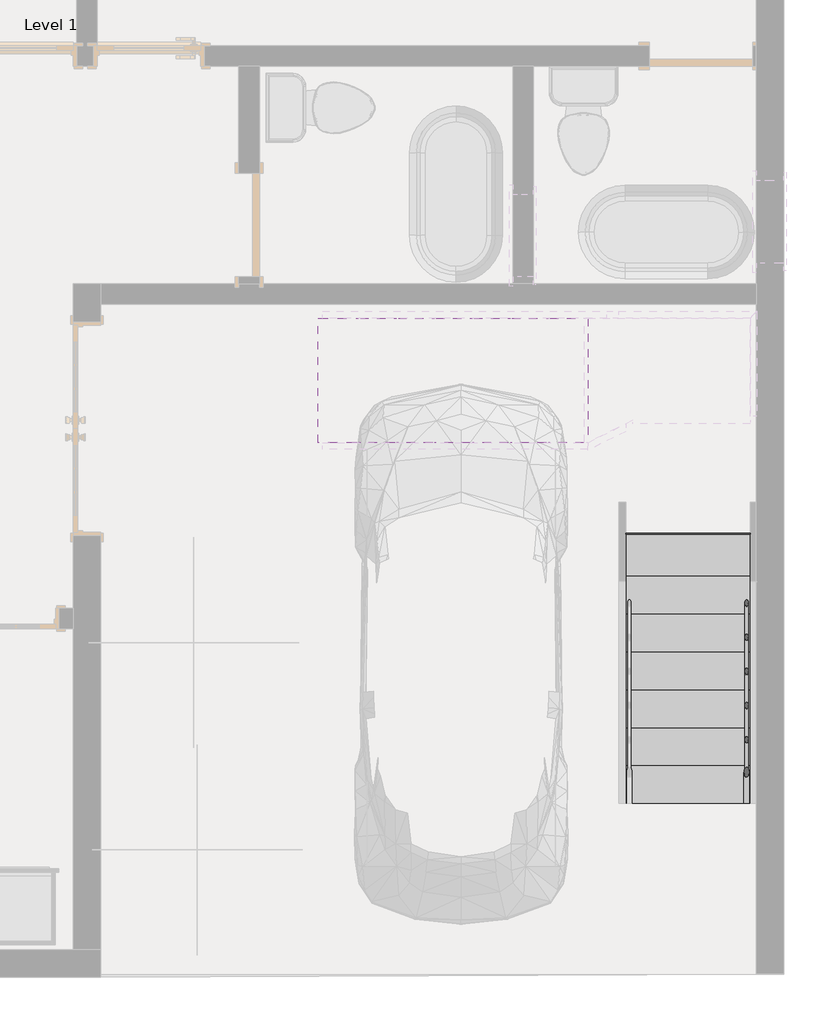
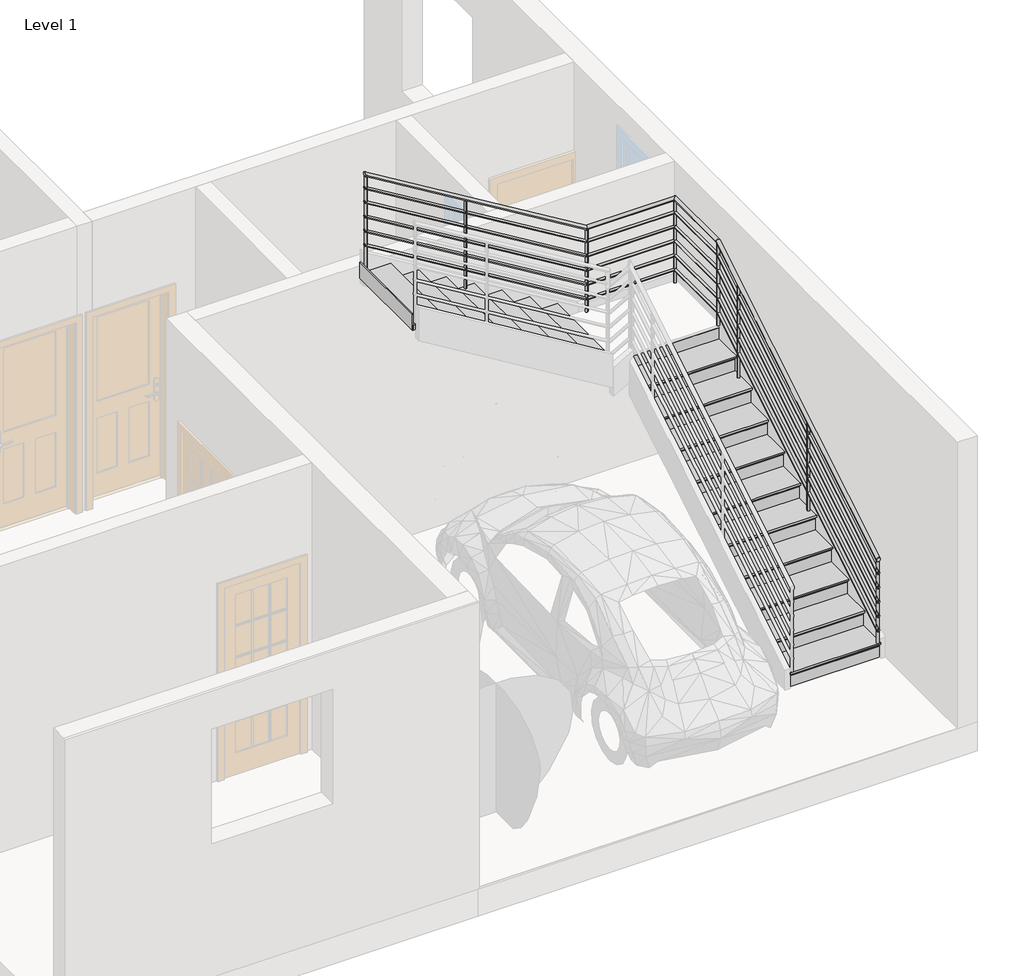
# One storey, part 4 of 5: 2 stair flights, 1 railing.
"""IFC4 building model written with IfcOpenShell, lengths in millimetres."""

from ifc_helpers import new_model, si_unit, point, frame, frame_2d, origin, place, context, project, spatial, circle_curve, ellipse_curve, trimmed, segment, composite_curve, outline, extrude, transform, mapped, element, save
from ifc_brep_helpers import plane_surface, cylinder_surface, advanced_brep
from components import stair_flight_5407f273, stair_flight_469bbda7

model = new_model("IFC4")

# Units and contexts
model_context = context("Model", 3, world=origin())
ifc_project = project(units=[si_unit("LENGTHUNIT", "METRE", prefix="MILLI")], contexts=[model_context])

# Site, building, storey
site = spatial("IfcSite", under=ifc_project)
building = spatial("IfcBuilding", under=site)
storey = spatial("IfcBuildingStorey", under=building, Name="Level 1", Elevation=0.0)

# Railing
placement = place(None, origin())
element("IfcRailing", 1, ObjectType="Handrail - Pipe", at=placement, inside=storey, context=model_context, shape_type="SolidModel", body=[
    advanced_brep(
    [(-1207.3432736, 3353.09939, 1061.4577857), (-1245.4432736, 3353.09939, 1061.4577857), (-4350.5932736, 6917.5700123, 4109.4577857), (-4350.5932736, 6879.4700123, 4109.4577857), (-1207.3432736, 6152.4215435, 2758.0166667), (-1245.4432736, 6152.4215435, 2758.0166667), (-1207.3432736, 6917.5700123, 2758.0166667), (-1245.4432736, 6879.4700123, 2758.0166667), (-2120.7154271, 6917.5700123, 2758.0166667), (-2120.7154271, 6879.4700123, 2758.0166667)],
    [
        (0, 1, ellipse_curve(frame((-1226.3932736, 3353.09939, 1061.4577857), z_axis=(0.0, -1.0, 0.0), x_axis=(0.0, 0.0, -1.0)), 22.2755476, 19.05)),
        (1, 0, ellipse_curve(frame((-1226.3932736, 3353.09939, 1061.4577857), z_axis=(0.0, -1.0, 0.0), x_axis=(0.0, 0.0, -1.0)), 22.2755476, 19.05)),
        (2, 3, ellipse_curve(frame((-4350.5932736, 6898.5200123, 4109.4577857), z_axis=(-1.0, 0.0, 0.0), x_axis=(0.0, 0.0, -1.0)), 22.2755476, 19.05)),
        (3, 2, ellipse_curve(frame((-4350.5932736, 6898.5200123, 4109.4577857), z_axis=(-1.0, 0.0, 0.0), x_axis=(0.0, 0.0, -1.0)), 22.2755476, 19.05)),
        (0, 4),
        (4, 5, ellipse_curve(frame((-1226.3932736, 6152.4215435, 2758.0166667), z_axis=(0.0, -0.9631193673564181, -0.26907449567540404), x_axis=(0.0, 0.26907449567540404, -0.963119367356418)), 19.7794797, 19.05)),
        (5, 1),
        (5, 4, ellipse_curve(frame((-1226.3932736, 6152.4215435, 2758.0166667), z_axis=(0.0, -0.9631193673564181, -0.26907449567540404), x_axis=(0.0, 0.26907449567540404, -0.963119367356418)), 19.7794797, 19.05)),
        (4, 6),
        (6, 7, ellipse_curve(frame((-1226.3932736, 6898.5200123, 2758.0166667), z_axis=(0.7071067811865457, -0.7071067811865495, 0.0), x_axis=(-0.7071067811865496, -0.7071067811865455, 0.0)), 26.9407684, 19.05)),
        (7, 5),
        (7, 6, ellipse_curve(frame((-1226.3932736, 6898.5200123, 2758.0166667), z_axis=(0.7071067811865457, -0.7071067811865495, 0.0), x_axis=(-0.7071067811865496, -0.7071067811865455, 0.0)), 26.9407684, 19.05)),
        (6, 8),
        (8, 9, ellipse_curve(frame((-2120.7154271, 6898.5200123, 2758.0166667), z_axis=(0.9631193673564181, 0.0, -0.2690744956754041), x_axis=(0.26907449567540354, 0.0, 0.9631193673564181)), 19.7794797, 19.05)),
        (9, 7),
        (9, 8, ellipse_curve(frame((-2120.7154271, 6898.5200123, 2758.0166667), z_axis=(0.9631193673564181, 0.0, -0.2690744956754041), x_axis=(0.26907449567540354, 0.0, 0.9631193673564181)), 19.7794797, 19.05)),
        (8, 2),
        (3, 9),
    ],
    [
        plane_surface(frame((-1226.3932736, 3353.09939, 1083.7333333), z_axis=(0.0, -1.0, 0.0), x_axis=(0.0, 0.0, 1.0))),
        plane_surface(frame((-4350.5932736, 6898.5200123, 4131.7333333), z_axis=(-1.0, 0.0, 0.0), x_axis=(0.0, -1.0, 0.0))),
        cylinder_surface(frame((-1226.3932736, 3362.9730377, 1067.4418146), z_axis=(0.0, -0.8551978315540542, -0.5183017160932847), x_axis=(-1.0, 0.0, 0.0)), 19.05),
        cylinder_surface(frame((-1226.3932736, 6147.09939, 2758.0166667), z_axis=(0.0, -1.0, 0.0), x_axis=(-1.0, 0.0, 0.0)), 19.05),
        cylinder_surface(frame((-1226.3932736, 6898.5200123, 2758.0166667), z_axis=(1.0, 0.0, 0.0), x_axis=(0.0, -1.0, 0.0)), 19.05),
        cylinder_surface(frame((-2125.2669212, 6898.5200123, 2760.775148), z_axis=(0.8551978315540539, 0.0, -0.5183017160932848), x_axis=(0.0, -1.0, 0.0)), 19.05),
    ],
    [
        (0, [[1, 2]]),
        (1, [[3, 4]]),
        (2, [[-1, 5, 6, 7]]),
        (2, [[-2, -7, 8, -5]]),
        (3, [[-6, 9, 10, 11]]),
        (3, [[-8, -11, 12, -9]]),
        (4, [[-10, 13, 14, 15]]),
        (4, [[-12, -15, 16, -13]]),
        (5, [[-14, 17, -4, 18]]),
        (5, [[-16, -18, -3, -17]]),
    ],
),
    advanced_brep(
    [(-1239.0932736, 3353.09939, 916.4829683), (-1213.6932736, 3353.09939, 916.4829683), (-1239.0932736, 6150.6474924, 2611.9666667), (-1213.6932736, 6150.6474924, 2611.9666667), (-1239.0932736, 6885.8200123, 2611.9666667), (-1213.6932736, 6911.2200123, 2611.9666667), (-2118.9413759, 6885.8200123, 2611.9666667), (-2118.9413759, 6911.2200123, 2611.9666667), (-4350.5932736, 6885.8200123, 3964.4829683), (-4350.5932736, 6911.2200123, 3964.4829683)],
    [
        (0, 1, ellipse_curve(frame((-1226.3932736, 3353.09939, 916.4829683), z_axis=(0.0, -1.0, 0.0), x_axis=(0.0, 0.0, -1.0)), 14.8503651, 12.7)),
        (1, 0, ellipse_curve(frame((-1226.3932736, 3353.09939, 916.4829683), z_axis=(0.0, -1.0, 0.0), x_axis=(0.0, 0.0, -1.0)), 14.8503651, 12.7)),
        (0, 2),
        (2, 3, ellipse_curve(frame((-1226.3932736, 6150.6474924, 2611.9666667), z_axis=(0.0, -0.9631193673564181, -0.26907449567540404), x_axis=(0.0, 0.26907449567540404, -0.963119367356418)), 13.1863198, 12.7)),
        (3, 1),
        (3, 2, ellipse_curve(frame((-1226.3932736, 6150.6474924, 2611.9666667), z_axis=(0.0, -0.9631193673564181, -0.26907449567540404), x_axis=(0.0, 0.26907449567540404, -0.963119367356418)), 13.1863198, 12.7)),
        (2, 4),
        (4, 5, ellipse_curve(frame((-1226.3932736, 6898.5200123, 2611.9666667), z_axis=(0.7071067811865457, -0.7071067811865495, 0.0), x_axis=(-0.7071067811865496, -0.7071067811865455, 0.0)), 17.9605122, 12.7)),
        (5, 3),
        (5, 4, ellipse_curve(frame((-1226.3932736, 6898.5200123, 2611.9666667), z_axis=(0.7071067811865457, -0.7071067811865495, 0.0), x_axis=(-0.7071067811865496, -0.7071067811865455, 0.0)), 17.9605122, 12.7)),
        (4, 6),
        (6, 7, ellipse_curve(frame((-2118.9413759, 6898.5200123, 2611.9666667), z_axis=(0.9631193673564181, 0.0, -0.2690744956754041), x_axis=(0.26907449567540354, 0.0, 0.9631193673564181)), 13.1863198, 12.7)),
        (7, 5),
        (7, 6, ellipse_curve(frame((-2118.9413759, 6898.5200123, 2611.9666667), z_axis=(0.9631193673564181, 0.0, -0.2690744956754041), x_axis=(0.26907449567540354, 0.0, 0.9631193673564181)), 13.1863198, 12.7)),
        (8, 9, ellipse_curve(frame((-4350.5932736, 6898.5200123, 3964.4829683), z_axis=(-1.0, 0.0, 0.0), x_axis=(0.0, 0.0, -1.0)), 14.8503651, 12.7)),
        (9, 8, ellipse_curve(frame((-4350.5932736, 6898.5200123, 3964.4829683), z_axis=(-1.0, 0.0, 0.0), x_axis=(0.0, 0.0, -1.0)), 14.8503651, 12.7)),
        (6, 8),
        (9, 7),
    ],
    [
        plane_surface(frame((-1226.3932736, 3353.09939, 931.3333333), z_axis=(0.0, -1.0, 0.0), x_axis=(0.0, 0.0, 1.0))),
        cylinder_surface(frame((-1226.3932736, 3359.6818218, 920.4723209), z_axis=(0.0, -0.8551978315540542, -0.5183017160932847), x_axis=(1.0, 0.0, 0.0)), 12.7),
        cylinder_surface(frame((-1226.3932736, 6147.09939, 2611.9666667), z_axis=(0.0, -1.0, 0.0), x_axis=(1.0, 0.0, 0.0)), 12.7),
        cylinder_surface(frame((-1226.3932736, 6898.5200123, 2611.9666667), z_axis=(1.0, 0.0, 0.0), x_axis=(0.0, 1.0, 0.0)), 12.7),
        plane_surface(frame((-4350.5932736, 6898.5200123, 3979.3333333), z_axis=(-1.0, 0.0, 0.0), x_axis=(0.0, -1.0, 0.0))),
        cylinder_surface(frame((-2121.9757054, 6898.5200123, 2613.8056542), z_axis=(0.8551978315540539, 0.0, -0.5183017160932848), x_axis=(0.0, 1.0, 0.0)), 12.7),
    ],
    [
        (0, [[1, 2]]),
        (1, [[-1, 3, 4, 5]]),
        (1, [[-2, -5, 6, -3]]),
        (2, [[-4, 7, 8, 9]]),
        (2, [[-6, -9, 10, -7]]),
        (3, [[-8, 11, 12, 13]]),
        (3, [[-10, -13, 14, -11]]),
        (4, [[15, 16]]),
        (5, [[-12, 17, -16, 18]]),
        (5, [[-14, -18, -15, -17]]),
    ],
),
    advanced_brep(
    [(-1239.0932736, 3353.09939, 764.0829683), (-1213.6932736, 3353.09939, 764.0829683), (-1239.0932736, 6150.6474924, 2459.5666667), (-1213.6932736, 6150.6474924, 2459.5666667), (-1239.0932736, 6885.8200123, 2459.5666667), (-1213.6932736, 6911.2200123, 2459.5666667), (-2118.9413759, 6885.8200123, 2459.5666667), (-2118.9413759, 6911.2200123, 2459.5666667), (-4350.5932736, 6885.8200123, 3812.0829683), (-4350.5932736, 6911.2200123, 3812.0829683)],
    [
        (0, 1, ellipse_curve(frame((-1226.3932736, 3353.09939, 764.0829683), z_axis=(0.0, -1.0, 0.0), x_axis=(0.0, 0.0, -1.0)), 14.8503651, 12.7)),
        (1, 0, ellipse_curve(frame((-1226.3932736, 3353.09939, 764.0829683), z_axis=(0.0, -1.0, 0.0), x_axis=(0.0, 0.0, -1.0)), 14.8503651, 12.7)),
        (0, 2),
        (2, 3, ellipse_curve(frame((-1226.3932736, 6150.6474924, 2459.5666667), z_axis=(0.0, -0.9631193673564181, -0.26907449567540404), x_axis=(0.0, 0.26907449567540404, -0.963119367356418)), 13.1863198, 12.7)),
        (3, 1),
        (3, 2, ellipse_curve(frame((-1226.3932736, 6150.6474924, 2459.5666667), z_axis=(0.0, -0.9631193673564181, -0.26907449567540404), x_axis=(0.0, 0.26907449567540404, -0.963119367356418)), 13.1863198, 12.7)),
        (2, 4),
        (4, 5, ellipse_curve(frame((-1226.3932736, 6898.5200123, 2459.5666667), z_axis=(0.7071067811865457, -0.7071067811865495, 0.0), x_axis=(-0.7071067811865496, -0.7071067811865455, 0.0)), 17.9605122, 12.7)),
        (5, 3),
        (5, 4, ellipse_curve(frame((-1226.3932736, 6898.5200123, 2459.5666667), z_axis=(0.7071067811865457, -0.7071067811865495, 0.0), x_axis=(-0.7071067811865496, -0.7071067811865455, 0.0)), 17.9605122, 12.7)),
        (4, 6),
        (6, 7, ellipse_curve(frame((-2118.9413759, 6898.5200123, 2459.5666667), z_axis=(0.9631193673564181, 0.0, -0.2690744956754041), x_axis=(0.26907449567540354, 0.0, 0.9631193673564181)), 13.1863198, 12.7)),
        (7, 5),
        (7, 6, ellipse_curve(frame((-2118.9413759, 6898.5200123, 2459.5666667), z_axis=(0.9631193673564181, 0.0, -0.2690744956754041), x_axis=(0.26907449567540354, 0.0, 0.9631193673564181)), 13.1863198, 12.7)),
        (8, 9, ellipse_curve(frame((-4350.5932736, 6898.5200123, 3812.0829683), z_axis=(-1.0, 0.0, 0.0), x_axis=(0.0, 0.0, -1.0)), 14.8503651, 12.7)),
        (9, 8, ellipse_curve(frame((-4350.5932736, 6898.5200123, 3812.0829683), z_axis=(-1.0, 0.0, 0.0), x_axis=(0.0, 0.0, -1.0)), 14.8503651, 12.7)),
        (6, 8),
        (9, 7),
    ],
    [
        plane_surface(frame((-1226.3932736, 3353.09939, 778.9333333), z_axis=(0.0, -1.0, 0.0), x_axis=(0.0, 0.0, 1.0))),
        cylinder_surface(frame((-1226.3932736, 3359.6818218, 768.0723209), z_axis=(0.0, -0.8551978315540542, -0.5183017160932847), x_axis=(1.0, 0.0, 0.0)), 12.7),
        cylinder_surface(frame((-1226.3932736, 6147.09939, 2459.5666667), z_axis=(0.0, -1.0, 0.0), x_axis=(1.0, 0.0, 0.0)), 12.7),
        cylinder_surface(frame((-1226.3932736, 6898.5200123, 2459.5666667), z_axis=(1.0, 0.0, 0.0), x_axis=(0.0, 1.0, 0.0)), 12.7),
        plane_surface(frame((-4350.5932736, 6898.5200123, 3826.9333333), z_axis=(-1.0, 0.0, 0.0), x_axis=(0.0, -1.0, 0.0))),
        cylinder_surface(frame((-2121.9757054, 6898.5200123, 2461.4056542), z_axis=(0.8551978315540539, 0.0, -0.5183017160932848), x_axis=(0.0, 1.0, 0.0)), 12.7),
    ],
    [
        (0, [[1, 2]]),
        (1, [[-1, 3, 4, 5]]),
        (1, [[-2, -5, 6, -3]]),
        (2, [[-4, 7, 8, 9]]),
        (2, [[-6, -9, 10, -7]]),
        (3, [[-8, 11, 12, 13]]),
        (3, [[-10, -13, 14, -11]]),
        (4, [[15, 16]]),
        (5, [[-12, 17, -16, 18]]),
        (5, [[-14, -18, -15, -17]]),
    ],
),
    advanced_brep(
    [(-1239.0932736, 3353.09939, 611.6829683), (-1213.6932736, 3353.09939, 611.6829683), (-1239.0932736, 6150.6474924, 2307.1666667), (-1213.6932736, 6150.6474924, 2307.1666667), (-1239.0932736, 6885.8200123, 2307.1666667), (-1213.6932736, 6911.2200123, 2307.1666667), (-2118.9413759, 6885.8200123, 2307.1666667), (-2118.9413759, 6911.2200123, 2307.1666667), (-4350.5932736, 6885.8200123, 3659.6829683), (-4350.5932736, 6911.2200123, 3659.6829683)],
    [
        (0, 1, ellipse_curve(frame((-1226.3932736, 3353.09939, 611.6829683), z_axis=(0.0, -1.0, 0.0), x_axis=(0.0, 0.0, -1.0)), 14.8503651, 12.7)),
        (1, 0, ellipse_curve(frame((-1226.3932736, 3353.09939, 611.6829683), z_axis=(0.0, -1.0, 0.0), x_axis=(0.0, 0.0, -1.0)), 14.8503651, 12.7)),
        (0, 2),
        (2, 3, ellipse_curve(frame((-1226.3932736, 6150.6474924, 2307.1666667), z_axis=(0.0, -0.9631193673564181, -0.269074495675404), x_axis=(0.0, 0.26907449567540426, -0.9631193673564179)), 13.1863198, 12.7)),
        (3, 1),
        (3, 2, ellipse_curve(frame((-1226.3932736, 6150.6474924, 2307.1666667), z_axis=(0.0, -0.9631193673564181, -0.269074495675404), x_axis=(0.0, 0.26907449567540426, -0.9631193673564179)), 13.1863198, 12.7)),
        (2, 4),
        (4, 5, ellipse_curve(frame((-1226.3932736, 6898.5200123, 2307.1666667), z_axis=(0.7071067811865457, -0.7071067811865495, 0.0), x_axis=(-0.7071067811865496, -0.7071067811865455, 0.0)), 17.9605122, 12.7)),
        (5, 3),
        (5, 4, ellipse_curve(frame((-1226.3932736, 6898.5200123, 2307.1666667), z_axis=(0.7071067811865457, -0.7071067811865495, 0.0), x_axis=(-0.7071067811865496, -0.7071067811865455, 0.0)), 17.9605122, 12.7)),
        (4, 6),
        (6, 7, ellipse_curve(frame((-2118.9413759, 6898.5200123, 2307.1666667), z_axis=(0.9631193673564181, 0.0, -0.269074495675404), x_axis=(0.26907449567540354, 0.0, 0.9631193673564181)), 13.1863198, 12.7)),
        (7, 5),
        (7, 6, ellipse_curve(frame((-2118.9413759, 6898.5200123, 2307.1666667), z_axis=(0.9631193673564181, 0.0, -0.269074495675404), x_axis=(0.26907449567540354, 0.0, 0.9631193673564181)), 13.1863198, 12.7)),
        (8, 9, ellipse_curve(frame((-4350.5932736, 6898.5200123, 3659.6829683), z_axis=(-1.0, 0.0, 0.0), x_axis=(0.0, 0.0, -1.0)), 14.8503651, 12.7)),
        (9, 8, ellipse_curve(frame((-4350.5932736, 6898.5200123, 3659.6829683), z_axis=(-1.0, 0.0, 0.0), x_axis=(0.0, 0.0, -1.0)), 14.8503651, 12.7)),
        (6, 8),
        (9, 7),
    ],
    [
        plane_surface(frame((-1226.3932736, 3353.09939, 626.5333333), z_axis=(0.0, -1.0, 0.0), x_axis=(0.0, 0.0, 1.0))),
        cylinder_surface(frame((-1226.3932736, 3359.6818218, 615.6723209), z_axis=(0.0, -0.855197831554054, -0.5183017160932847), x_axis=(1.0, 0.0, 0.0)), 12.7),
        cylinder_surface(frame((-1226.3932736, 6147.09939, 2307.1666667), z_axis=(0.0, -1.0, 0.0), x_axis=(1.0, 0.0, 0.0)), 12.7),
        cylinder_surface(frame((-1226.3932736, 6898.5200123, 2307.1666667), z_axis=(1.0, 0.0, 0.0), x_axis=(0.0, 1.0, 0.0)), 12.7),
        plane_surface(frame((-4350.5932736, 6898.5200123, 3674.5333333), z_axis=(-1.0, 0.0, 0.0), x_axis=(0.0, -1.0, 0.0))),
        cylinder_surface(frame((-2121.9757054, 6898.5200123, 2309.0056542), z_axis=(0.855197831554054, 0.0, -0.5183017160932847), x_axis=(0.0, 1.0, 0.0)), 12.7),
    ],
    [
        (0, [[1, 2]]),
        (1, [[-1, 3, 4, 5]]),
        (1, [[-2, -5, 6, -3]]),
        (2, [[-4, 7, 8, 9]]),
        (2, [[-6, -9, 10, -7]]),
        (3, [[-8, 11, 12, 13]]),
        (3, [[-10, -13, 14, -11]]),
        (4, [[15, 16]]),
        (5, [[-12, 17, -16, 18]]),
        (5, [[-14, -18, -15, -17]]),
    ],
),
    advanced_brep(
    [(-1239.0932736, 3353.09939, 459.2829683), (-1213.6932736, 3353.09939, 459.2829683), (-1239.0932736, 6150.6474924, 2154.7666667), (-1213.6932736, 6150.6474924, 2154.7666667), (-1239.0932736, 6885.8200123, 2154.7666667), (-1213.6932736, 6911.2200123, 2154.7666667), (-2118.9413759, 6885.8200123, 2154.7666667), (-2118.9413759, 6911.2200123, 2154.7666667), (-4350.5932736, 6885.8200123, 3507.2829683), (-4350.5932736, 6911.2200123, 3507.2829683)],
    [
        (0, 1, ellipse_curve(frame((-1226.3932736, 3353.09939, 459.2829683), z_axis=(0.0, -1.0, 0.0), x_axis=(0.0, 0.0, -1.0)), 14.8503651, 12.7)),
        (1, 0, ellipse_curve(frame((-1226.3932736, 3353.09939, 459.2829683), z_axis=(0.0, -1.0, 0.0), x_axis=(0.0, 0.0, -1.0)), 14.8503651, 12.7)),
        (0, 2),
        (2, 3, ellipse_curve(frame((-1226.3932736, 6150.6474924, 2154.7666667), z_axis=(0.0, -0.9631193673564181, -0.269074495675404), x_axis=(0.0, 0.26907449567540426, -0.9631193673564179)), 13.1863198, 12.7)),
        (3, 1),
        (3, 2, ellipse_curve(frame((-1226.3932736, 6150.6474924, 2154.7666667), z_axis=(0.0, -0.9631193673564181, -0.269074495675404), x_axis=(0.0, 0.26907449567540426, -0.9631193673564179)), 13.1863198, 12.7)),
        (2, 4),
        (4, 5, ellipse_curve(frame((-1226.3932736, 6898.5200123, 2154.7666667), z_axis=(0.7071067811865457, -0.7071067811865495, 0.0), x_axis=(-0.7071067811865496, -0.7071067811865455, 0.0)), 17.9605122, 12.7)),
        (5, 3),
        (5, 4, ellipse_curve(frame((-1226.3932736, 6898.5200123, 2154.7666667), z_axis=(0.7071067811865457, -0.7071067811865495, 0.0), x_axis=(-0.7071067811865496, -0.7071067811865455, 0.0)), 17.9605122, 12.7)),
        (4, 6),
        (6, 7, ellipse_curve(frame((-2118.9413759, 6898.5200123, 2154.7666667), z_axis=(0.9631193673564181, 0.0, -0.269074495675404), x_axis=(0.26907449567540354, 0.0, 0.9631193673564181)), 13.1863198, 12.7)),
        (7, 5),
        (7, 6, ellipse_curve(frame((-2118.9413759, 6898.5200123, 2154.7666667), z_axis=(0.9631193673564181, 0.0, -0.269074495675404), x_axis=(0.26907449567540354, 0.0, 0.9631193673564181)), 13.1863198, 12.7)),
        (8, 9, ellipse_curve(frame((-4350.5932736, 6898.5200123, 3507.2829683), z_axis=(-1.0, 0.0, 0.0), x_axis=(0.0, 0.0, -1.0)), 14.8503651, 12.7)),
        (9, 8, ellipse_curve(frame((-4350.5932736, 6898.5200123, 3507.2829683), z_axis=(-1.0, 0.0, 0.0), x_axis=(0.0, 0.0, -1.0)), 14.8503651, 12.7)),
        (6, 8),
        (9, 7),
    ],
    [
        plane_surface(frame((-1226.3932736, 3353.09939, 474.1333333), z_axis=(0.0, -1.0, 0.0), x_axis=(0.0, 0.0, 1.0))),
        cylinder_surface(frame((-1226.3932736, 3359.6818218, 463.2723209), z_axis=(0.0, -0.855197831554054, -0.5183017160932847), x_axis=(1.0, 0.0, 0.0)), 12.7),
        cylinder_surface(frame((-1226.3932736, 6147.09939, 2154.7666667), z_axis=(0.0, -1.0, 0.0), x_axis=(1.0, 0.0, 0.0)), 12.7),
        cylinder_surface(frame((-1226.3932736, 6898.5200123, 2154.7666667), z_axis=(1.0, 0.0, 0.0), x_axis=(0.0, 1.0, 0.0)), 12.7),
        plane_surface(frame((-4350.5932736, 6898.5200123, 3522.1333333), z_axis=(-1.0, 0.0, 0.0), x_axis=(0.0, -1.0, 0.0))),
        cylinder_surface(frame((-2121.9757054, 6898.5200123, 2156.6056542), z_axis=(0.855197831554054, 0.0, -0.5183017160932847), x_axis=(0.0, 1.0, 0.0)), 12.7),
    ],
    [
        (0, [[1, 2]]),
        (1, [[-1, 3, 4, 5]]),
        (1, [[-2, -5, 6, -3]]),
        (2, [[-4, 7, 8, 9]]),
        (2, [[-6, -9, 10, -7]]),
        (3, [[-8, 11, 12, 13]]),
        (3, [[-10, -13, 14, -11]]),
        (4, [[15, 16]]),
        (5, [[-12, 17, -16, 18]]),
        (5, [[-14, -18, -15, -17]]),
    ],
),
    advanced_brep(
    [(-1239.0932736, 3353.09939, 306.8829683), (-1213.6932736, 3353.09939, 306.8829683), (-1239.0932736, 6150.6474924, 2002.3666667), (-1213.6932736, 6150.6474924, 2002.3666667), (-1239.0932736, 6885.8200123, 2002.3666667), (-1213.6932736, 6911.2200123, 2002.3666667), (-2118.9413759, 6885.8200123, 2002.3666667), (-2118.9413759, 6911.2200123, 2002.3666667), (-4350.5932736, 6885.8200123, 3354.8829683), (-4350.5932736, 6911.2200123, 3354.8829683)],
    [
        (0, 1, ellipse_curve(frame((-1226.3932736, 3353.09939, 306.8829683), z_axis=(0.0, -1.0, 0.0), x_axis=(0.0, 0.0, -1.0)), 14.8503651, 12.7)),
        (1, 0, ellipse_curve(frame((-1226.3932736, 3353.09939, 306.8829683), z_axis=(0.0, -1.0, 0.0), x_axis=(0.0, 0.0, -1.0)), 14.8503651, 12.7)),
        (0, 2),
        (2, 3, ellipse_curve(frame((-1226.3932736, 6150.6474924, 2002.3666667), z_axis=(0.0, -0.9631193673564181, -0.269074495675404), x_axis=(0.0, 0.26907449567540426, -0.9631193673564179)), 13.1863198, 12.7)),
        (3, 1),
        (3, 2, ellipse_curve(frame((-1226.3932736, 6150.6474924, 2002.3666667), z_axis=(0.0, -0.9631193673564181, -0.269074495675404), x_axis=(0.0, 0.26907449567540426, -0.9631193673564179)), 13.1863198, 12.7)),
        (2, 4),
        (4, 5, ellipse_curve(frame((-1226.3932736, 6898.5200123, 2002.3666667), z_axis=(0.7071067811865457, -0.7071067811865495, 0.0), x_axis=(-0.7071067811865496, -0.7071067811865455, 0.0)), 17.9605122, 12.7)),
        (5, 3),
        (5, 4, ellipse_curve(frame((-1226.3932736, 6898.5200123, 2002.3666667), z_axis=(0.7071067811865457, -0.7071067811865495, 0.0), x_axis=(-0.7071067811865496, -0.7071067811865455, 0.0)), 17.9605122, 12.7)),
        (4, 6),
        (6, 7, ellipse_curve(frame((-2118.9413759, 6898.5200123, 2002.3666667), z_axis=(0.9631193673564181, 0.0, -0.269074495675404), x_axis=(0.26907449567540354, 0.0, 0.9631193673564181)), 13.1863198, 12.7)),
        (7, 5),
        (7, 6, ellipse_curve(frame((-2118.9413759, 6898.5200123, 2002.3666667), z_axis=(0.9631193673564181, 0.0, -0.269074495675404), x_axis=(0.26907449567540354, 0.0, 0.9631193673564181)), 13.1863198, 12.7)),
        (8, 9, ellipse_curve(frame((-4350.5932736, 6898.5200123, 3354.8829683), z_axis=(-1.0, 0.0, 0.0), x_axis=(0.0, 0.0, -1.0)), 14.8503651, 12.7)),
        (9, 8, ellipse_curve(frame((-4350.5932736, 6898.5200123, 3354.8829683), z_axis=(-1.0, 0.0, 0.0), x_axis=(0.0, 0.0, -1.0)), 14.8503651, 12.7)),
        (6, 8),
        (9, 7),
    ],
    [
        plane_surface(frame((-1226.3932736, 3353.09939, 321.7333333), z_axis=(0.0, -1.0, 0.0), x_axis=(0.0, 0.0, 1.0))),
        cylinder_surface(frame((-1226.3932736, 3359.6818218, 310.8723209), z_axis=(0.0, -0.855197831554054, -0.5183017160932847), x_axis=(1.0, 0.0, 0.0)), 12.7),
        cylinder_surface(frame((-1226.3932736, 6147.09939, 2002.3666667), z_axis=(0.0, -1.0, 0.0), x_axis=(1.0, 0.0, 0.0)), 12.7),
        cylinder_surface(frame((-1226.3932736, 6898.5200123, 2002.3666667), z_axis=(1.0, 0.0, 0.0), x_axis=(0.0, 1.0, 0.0)), 12.7),
        plane_surface(frame((-4350.5932736, 6898.5200123, 3369.7333333), z_axis=(-1.0, 0.0, 0.0), x_axis=(0.0, -1.0, 0.0))),
        cylinder_surface(frame((-2121.9757054, 6898.5200123, 2004.2056542), z_axis=(0.855197831554054, 0.0, -0.5183017160932847), x_axis=(0.0, 1.0, 0.0)), 12.7),
    ],
    [
        (0, [[1, 2]]),
        (1, [[-1, 3, 4, 5]]),
        (1, [[-2, -5, 6, -3]]),
        (2, [[-4, 7, 8, 9]]),
        (2, [[-6, -9, 10, -7]]),
        (3, [[-8, 11, 12, 13]]),
        (3, [[-10, -13, 14, -11]]),
        (4, [[15, 16]]),
        (5, [[-12, 17, -16, 18]]),
        (5, [[-14, -18, -15, -17]]),
    ],
),
    advanced_brep(
    [(-3334.5932736, 6911.2200123, 3471.4246624), (-3334.5932736, 6911.2200123, 2540.0), (-3334.5932736, 6885.8200123, 2540.0), (-3334.5932736, 6885.8200123, 3471.4246624)],
    [
        (0, 1),
        (1, 2, circle_curve(frame((-3334.5932736, 6898.5200123, 2540.0), z_axis=(0.0, 0.0, 1.0), x_axis=(0.0, -1.0, 0.0)), 12.7)),
        (2, 3),
        (3, 0, ellipse_curve(frame((-3334.5932736, 6898.5200123, 3471.4246624), z_axis=(-0.5183017160932849, 0.0, -0.8551978315540538), x_axis=(-0.8551978315540538, 0.0, 0.518301716093285)), 14.8503651, 12.7)),
        (0, 3, ellipse_curve(frame((-3334.5932736, 6898.5200123, 3471.4246624), z_axis=(-0.5183017160932849, 0.0, -0.8551978315540538), x_axis=(-0.8551978315540538, 0.0, 0.518301716093285)), 14.8503651, 12.7)),
        (2, 1, circle_curve(frame((-3334.5932736, 6898.5200123, 2540.0), z_axis=(0.0, 0.0, 1.0), x_axis=(0.0, -1.0, 0.0)), 12.7)),
    ],
    [
        cylinder_surface(frame((-3334.5932736, 6898.5200123, 2311.4), z_axis=(0.0, 0.0, 1.0), x_axis=(0.0, -1.0, 0.0)), 12.7),
        plane_surface(frame((-3359.9932736, 6873.1200123, 3486.8186018), z_axis=(0.5183017160932849, 0.0, 0.8551978315540538), x_axis=(0.0, 1.0, 0.0))),
        plane_surface(frame((-3309.1932736, 6873.1200123, 2540.0), z_axis=(0.0, 0.0, -1.0), x_axis=(0.0, 1.0, 0.0))),
    ],
    [
        (0, [[1, 2, 3, 4]]),
        (0, [[-1, 5, -3, 6]]),
        (1, [[-4, -5]]),
        (2, [[-2, -6]]),
    ],
),
    advanced_brep(
    [(-1213.6932736, 5791.49939, 2517.00042), (-1213.6932736, 5791.49939, 1524.0), (-1239.0932736, 5791.49939, 1524.0), (-1239.0932736, 5791.49939, 2517.00042)],
    [
        (0, 1),
        (1, 2, circle_curve(frame((-1226.3932736, 5791.49939, 1524.0), z_axis=(0.0, 0.0, 1.0), x_axis=(-1.0, 0.0, 0.0)), 12.7)),
        (2, 3),
        (3, 0, ellipse_curve(frame((-1226.3932736, 5791.49939, 2517.00042), z_axis=(0.0, 0.5183017160932833, -0.8551978315540549), x_axis=(0.0, 0.855197831554055, 0.518301716093283)), 14.8503651, 12.7)),
        (0, 3, ellipse_curve(frame((-1226.3932736, 5791.49939, 2517.00042), z_axis=(0.0, 0.5183017160932833, -0.8551978315540549), x_axis=(0.0, 0.855197831554055, 0.518301716093283)), 14.8503651, 12.7)),
        (2, 1, circle_curve(frame((-1226.3932736, 5791.49939, 1524.0), z_axis=(0.0, 0.0, 1.0), x_axis=(-1.0, 0.0, 0.0)), 12.7)),
    ],
    [
        cylinder_surface(frame((-1226.3932736, 5791.49939, 1295.4), z_axis=(0.0, 0.0, 1.0), x_axis=(-1.0, 0.0, 0.0)), 12.7),
        plane_surface(frame((-1251.7932736, 5816.89939, 2532.3943594), z_axis=(0.0, -0.5183017160932833, 0.8551978315540549), x_axis=(1.0, 0.0, 0.0))),
        plane_surface(frame((-1251.7932736, 5766.09939, 1524.0), z_axis=(0.0, 0.0, -1.0), x_axis=(1.0, 0.0, 0.0))),
    ],
    [
        (0, [[1, 2, 3, 4]]),
        (0, [[-1, 5, -3, 6]]),
        (1, [[-4, -5]]),
        (2, [[-2, -6]]),
    ],
),
    advanced_brep(
    [(-1213.6932736, 4572.29939, 1778.0913291), (-1213.6932736, 4572.29939, 846.6666667), (-1239.0932736, 4572.29939, 846.6666667), (-1239.0932736, 4572.29939, 1778.0913291)],
    [
        (0, 1),
        (1, 2, circle_curve(frame((-1226.3932736, 4572.29939, 846.6666667), z_axis=(0.0, 0.0, 1.0), x_axis=(-1.0, 0.0, 0.0)), 12.7)),
        (2, 3),
        (3, 0, ellipse_curve(frame((-1226.3932736, 4572.29939, 1778.0913291), z_axis=(0.0, 0.5183017160932849, -0.8551978315540538), x_axis=(0.0, 0.8551978315540538, 0.518301716093285)), 14.8503651, 12.7)),
        (0, 3, ellipse_curve(frame((-1226.3932736, 4572.29939, 1778.0913291), z_axis=(0.0, 0.5183017160932849, -0.8551978315540538), x_axis=(0.0, 0.8551978315540538, 0.518301716093285)), 14.8503651, 12.7)),
        (2, 1, circle_curve(frame((-1226.3932736, 4572.29939, 846.6666667), z_axis=(0.0, 0.0, 1.0), x_axis=(-1.0, 0.0, 0.0)), 12.7)),
    ],
    [
        cylinder_surface(frame((-1226.3932736, 4572.29939, 618.0666667), z_axis=(0.0, 0.0, 1.0), x_axis=(-1.0, 0.0, 0.0)), 12.7),
        plane_surface(frame((-1251.7932736, 4597.69939, 1793.4852684), z_axis=(0.0, -0.5183017160932849, 0.8551978315540538), x_axis=(1.0, 0.0, 0.0))),
        plane_surface(frame((-1251.7932736, 4546.89939, 846.6666667), z_axis=(0.0, 0.0, -1.0), x_axis=(1.0, 0.0, 0.0))),
    ],
    [
        (0, [[1, 2, 3, 4]]),
        (0, [[-1, 5, -3, 6]]),
        (1, [[-4, -5]]),
        (2, [[-2, -6]]),
    ],
),
    extrude(outline(composite_curve([segment(trimmed(circle_curve(frame_2d((-2115.3932736, 6898.5200123)), 12.7), [point((-2115.3932736, 6885.8200123))], [point((-2115.3932736, 6911.2200123))], False, "CARTESIAN"), True, "CONTINUOUS"), segment(trimmed(circle_curve(frame_2d((-2115.3932736, 6898.5200123)), 12.7), [point((-2115.3932736, 6911.2200123))], [point((-2115.3932736, 6885.8200123))], False, "CARTESIAN"), True, "CONTINUOUS")], self_intersect=False)), frame((0.0, 0.0, 1862.6666667), z_axis=(0.0, 0.0, 1.0), x_axis=(1.0, 0.0, 0.0)), (0.0, 0.0, 1.0), 876.3),
    extrude(outline(composite_curve([segment(trimmed(circle_curve(frame_2d((-1226.3932736, 6898.5200123)), 12.7), [point((-1239.0932736, 6898.5200123))], [point((-1213.6932736, 6898.5200123))], False, "CARTESIAN"), True, "CONTINUOUS"), segment(trimmed(circle_curve(frame_2d((-1226.3932736, 6898.5200123)), 12.7), [point((-1213.6932736, 6898.5200123))], [point((-1239.0932736, 6898.5200123))], False, "CARTESIAN"), True, "CONTINUOUS")], self_intersect=False)), frame((0.0, 0.0, 1862.6666667), z_axis=(0.0, 0.0, 1.0), x_axis=(1.0, 0.0, 0.0)), (0.0, 0.0, 1.0), 876.3),
    extrude(outline(composite_curve([segment(trimmed(circle_curve(frame_2d((-1226.3932736, 6147.09939)), 12.7), [point((-1239.0932736, 6147.09939))], [point((-1213.6932736, 6147.09939))], False, "CARTESIAN"), True, "CONTINUOUS"), segment(trimmed(circle_curve(frame_2d((-1226.3932736, 6147.09939)), 12.7), [point((-1213.6932736, 6147.09939))], [point((-1239.0932736, 6147.09939))], False, "CARTESIAN"), True, "CONTINUOUS")], self_intersect=False)), frame((0.0, 0.0, 1862.6666667), z_axis=(0.0, 0.0, 1.0), x_axis=(1.0, 0.0, 0.0)), (0.0, 0.0, 1.0), 876.3),
    advanced_brep(
    [(-4337.8932736, 6911.2200123, 4079.4852684), (-4337.8932736, 6911.2200123, 3048.0), (-4337.8932736, 6885.8200123, 3048.0), (-4337.8932736, 6885.8200123, 4079.4852684)],
    [
        (0, 1),
        (1, 2, circle_curve(frame((-4337.8932736, 6898.5200123, 3048.0), z_axis=(0.0, 0.0, 1.0), x_axis=(0.0, -1.0, 0.0)), 12.7)),
        (2, 3),
        (3, 0, ellipse_curve(frame((-4337.8932736, 6898.5200123, 4079.4852684), z_axis=(-0.5183017160932833, 0.0, -0.8551978315540549), x_axis=(-0.855197831554055, 0.0, 0.518301716093283)), 14.8503651, 12.7)),
        (0, 3, ellipse_curve(frame((-4337.8932736, 6898.5200123, 4079.4852684), z_axis=(-0.5183017160932833, 0.0, -0.8551978315540549), x_axis=(-0.855197831554055, 0.0, 0.518301716093283)), 14.8503651, 12.7)),
        (2, 1, circle_curve(frame((-4337.8932736, 6898.5200123, 3048.0), z_axis=(0.0, 0.0, 1.0), x_axis=(0.0, -1.0, 0.0)), 12.7)),
    ],
    [
        cylinder_surface(frame((-4337.8932736, 6898.5200123, 2819.4), z_axis=(0.0, 0.0, 1.0), x_axis=(0.0, -1.0, 0.0)), 12.7),
        plane_surface(frame((-4363.2932736, 6873.1200123, 4094.8792078), z_axis=(0.5183017160932833, 0.0, 0.8551978315540549), x_axis=(0.0, 1.0, 0.0))),
        plane_surface(frame((-4312.4932736, 6873.1200123, 3048.0), z_axis=(0.0, 0.0, -1.0), x_axis=(0.0, 1.0, 0.0))),
    ],
    [
        (0, [[1, 2, 3, 4]]),
        (0, [[-1, 5, -3, 6]]),
        (1, [[-4, -5]]),
        (2, [[-2, -6]]),
    ],
),
    advanced_brep(
    [(-1213.6932736, 3365.79939, 1046.8792078), (-1213.6932736, 3365.79939, 169.3333333), (-1239.0932736, 3365.79939, 169.3333333), (-1239.0932736, 3365.79939, 1046.8792078)],
    [
        (0, 1),
        (1, 2, circle_curve(frame((-1226.3932736, 3365.79939, 169.3333333), z_axis=(0.0, 0.0, 1.0), x_axis=(-1.0, 0.0, 0.0)), 12.7)),
        (2, 3),
        (3, 0, ellipse_curve(frame((-1226.3932736, 3365.79939, 1046.8792078), z_axis=(0.0, 0.5183017160932833, -0.8551978315540549), x_axis=(0.0, 0.855197831554055, 0.518301716093283)), 14.8503651, 12.7)),
        (0, 3, ellipse_curve(frame((-1226.3932736, 3365.79939, 1046.8792078), z_axis=(0.0, 0.5183017160932833, -0.8551978315540549), x_axis=(0.0, 0.855197831554055, 0.518301716093283)), 14.8503651, 12.7)),
        (2, 1, circle_curve(frame((-1226.3932736, 3365.79939, 169.3333333), z_axis=(0.0, 0.0, 1.0), x_axis=(-1.0, 0.0, 0.0)), 12.7)),
    ],
    [
        cylinder_surface(frame((-1226.3932736, 3365.79939, -59.2666667), z_axis=(0.0, 0.0, 1.0), x_axis=(-1.0, 0.0, 0.0)), 12.7),
        plane_surface(frame((-1251.7932736, 3391.19939, 1062.2731472), z_axis=(0.0, -0.5183017160932833, 0.8551978315540549), x_axis=(1.0, 0.0, 0.0))),
        plane_surface(frame((-1251.7932736, 3340.39939, 169.3333333), z_axis=(0.0, 0.0, -1.0), x_axis=(1.0, 0.0, 0.0))),
    ],
    [
        (0, [[1, 2, 3, 4]]),
        (0, [[-1, 5, -3, 6]]),
        (1, [[-4, -5]]),
        (2, [[-2, -6]]),
    ],
),
])

# Stair flights
stair_flight_shape = stair_flight_5407f273(model_context)
element("IfcStairFlight", 2, ObjectType="2\" Tread 1\" Nosing 1/4\" Riser", at=placement, inside=storey, context=model_context, shape_type="MappedRepresentation", body=[
    mapped(stair_flight_shape, transform((0.0, 0.0, 0.0), x_axis=(1.0, 0.0, 0.0), y_axis=(0.0, 1.0, 0.0), z_axis=(0.0, 0.0, 1.0))),
])
stair_flight_2_shape = stair_flight_469bbda7(model_context)
element("IfcStairFlight", 3, ObjectType="2\" Tread 1\" Nosing 1/4\" Riser", at=placement, inside=storey, context=model_context, shape_type="MappedRepresentation", body=[
    mapped(stair_flight_2_shape, transform((0.0, 0.0, 0.0), x_axis=(1.0, 0.0, 0.0), y_axis=(0.0, 1.0, 0.0), z_axis=(0.0, 0.0, 1.0))),
])

save(model, "model.ifc")

# Revit data of these elements
# Type "Handrail - Pipe"
#   Assembly Code = "C2010400"
#   built-in parameter 1008612 = 0.0416667 (stored number, unit not read)
#   built-in parameter 1008611 = 0.0833333 (stored number, unit not read)
#   built-in parameter 1008609 = 4 (stored number, unit not read)
#   built-in parameter 1008604 = 0.166667 (stored number, unit not read)
#   built-in parameter 1008603 = 0.166667 (stored number, unit not read)
#   Railing Height = 3' - 0"
#   built-in parameter 1008630 = 2
#   built-in parameter 1008610 = 1
#   built-in parameter 1008605 = 1
#   built-in parameter 1008618 = Baluster - Round : 1"
# Element 1 (IfcRailing, "Handrail - Pipe")
#   Phase Created = New Construction
# Elements 2, 3 (IfcStairFlight, "2\" Tread 1\" Nosing 1/4\" Riser")
#   Phase Created = New Construction
